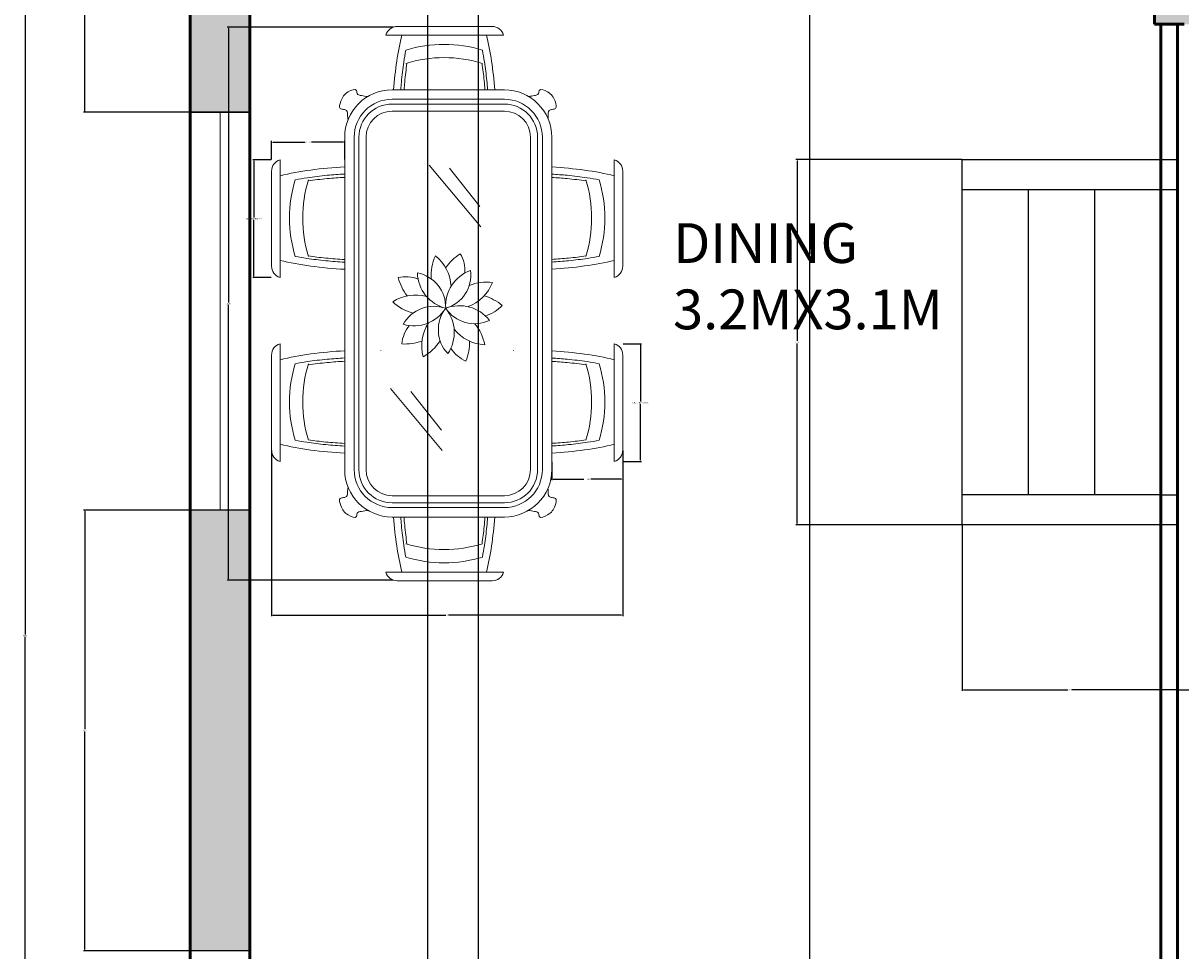
# Model space of a CAD drawing. Units: inches. Extents: x 3 to 380, y -485 to 60.
# Tile 4 of 8: x 3 to 177, y -270 to -130. Entities that reach past the tile are written whole.
import ezdxf

# ---------------------------------------------------------------- set-up
doc = ezdxf.new("R2010")
doc.units = ezdxf.units.IN
doc.header["$MEASUREMENT"] = 0
for name, color, linetype, lineweight in [('A-ANNO-DIMS', 2, 'Continuous', 18), ('A-AREA-IDEN', 7, 'Continuous', 25), ('A-FLOR-STRS', 7, 'Continuous', 25), ('A-FURN', 8, 'Continuous', 18), ('A-GLAZ', 4, 'Continuous', 18), ('A-WALL', 7, 'Continuous', 50), ('A-WALL-PATT', 252, 'Continuous', 13)]:
    doc.layers.add(name, color=color, linetype=linetype, lineweight=lineweight)
doc.styles.get("Standard").update_dxf_attribs({"font": 'arial.ttf'})
doc.dimstyles.get("Standard").update_dxf_attribs({"dimtxt": 0.18, "dimasz": 0.18, "dimexe": 0.18, "dimexo": 0.0625, "dimgap": 0.09, "dimtad": 0, "dimtih": 1, "dimtoh": 1, "dimdec": 0, "dimzin": 0, "dimdsep": 46, "dimlunit": 3, "dimtxsty": 'Standard', "dimcen": 0.09, "dimadec": 0, "dimazin": 0, "dimtfac": 1, "dimtdec": 0, "dimtofl": 0, "dimtmove": 0, "dimatfit": 3, "dimfxl": 1, "dimtolj": 1, "dimtzin": 0, "dimarcsym": 0})

# ---------------------------------------------------------------- blocks, each defined once
blk = doc.blocks.new('WIN-60X9')
for p, q in [((60, 9), (0, 9)), ((0, 9), (0, 0)), ((60, 0), (60, 9)), ((0, 4.5), (60, 4.5)), ((0, 0), (60, 0))]:
    blk.add_line(p, q)
blk = doc.blocks.new('DINING-CHAIR-A')
blk.add_line((9.42, 0), (9.42, 17.76))
blk.add_lwpolyline([(9.42, 17.76, -0.333667), (10.71, 16.04), (10.71, 1.72, -0.333667), (9.42, 0)], format="xyb")
for centre in [(-13.43, 8.97), (-11.43, 8.97)]:
    blk.add_arc(centre, 19.44, 342.7033, 17.2967)
at = {"extrusion": (0, 0, -1)}
for start_param, end_param in [(1.730141, 2.183659), (4.099527, 4.553045)]:
    blk.add_ellipse((-3.59, 8.97), major_axis=(-22.61, 0), ratio=0.345133, start_param=start_param, end_param=end_param, dxfattribs=at)
for points, knots in [([(0, 15.6), (0.78, 15.55), (1.55, 15.49), (3.34, 15.32), (4.35, 15.2), (5.94, 14.96), (6.54, 14.86), (7.13, 14.75)], [8.0160361, 8.0160361, 8.0160361, 8.0160361, 8.1227425, 8.1227425, 8.2664644, 8.2664644, 8.3579144, 8.3579144, 8.3579144, 8.3579144]), ([(0, 15.1), (0.78, 15.05), (1.55, 14.99), (3.29, 14.83), (4.25, 14.71), (5.18, 14.57)], [8.0160361, 8.0160361, 8.0160361, 8.0160361, 8.1227425, 8.1227425, 8.2598231, 8.2598231, 8.2598231, 8.2598231]), ([(5.15, 3.25), (4.3, 3.13), (3.43, 3.02), (1.7, 2.85), (0.86, 2.78), (0, 2.74)], [4.3081151, 4.3081151, 4.3081151, 4.3081151, 4.433179, 4.433179, 4.5503345, 4.5503345, 4.5503345, 4.5503345]), ([(7.13, 3.19), (6.56, 3.08), (5.98, 2.98), (4.47, 2.75), (3.51, 2.63), (1.7, 2.45), (0.86, 2.38), (0, 2.34)], [4.2084563, 4.2084563, 4.2084563, 4.2084563, 4.2962292, 4.2962292, 4.433179, 4.433179, 4.5503345, 4.5503345, 4.5503345, 4.5503345])]:
    blk.add_open_spline(points, degree=3, knots=knots)
blk = doc.blocks.new('DINING-CHAIR-B')
blk.add_line((1.29, 0), (1.29, 17.76))
blk.add_lwpolyline([(1.29, 17.76, 0.333667), (0, 16.04), (0, 1.72, 0.333667), (1.29, 0)], format="xyb")
for centre in [(22.14, 8.97), (24.14, 8.97)]:
    blk.add_arc(centre, 19.44, 162.7033, 197.2967)
for start_param, end_param in [(7.99879, 8.466844), (4.099527, 4.56758)]:
    blk.add_ellipse((14.3, 8.97), major_axis=(22.61, 0), ratio=0.345133, start_param=start_param, end_param=end_param)
for points, knots in [([(11.04, 15.61), (10.14, 15.57), (9.26, 15.5), (7.37, 15.32), (6.37, 15.2), (4.78, 14.96), (4.17, 14.86), (3.58, 14.75)], [8.0012444, 8.0012444, 8.0012444, 8.0012444, 8.1227425, 8.1227425, 8.2664644, 8.2664644, 8.3579144, 8.3579144, 8.3579144, 8.3579144]), ([(11.04, 15.11), (10.14, 15.07), (9.26, 15), (7.42, 14.83), (6.46, 14.71), (5.53, 14.57)], [8.0012444, 8.0012444, 8.0012444, 8.0012444, 8.1227425, 8.1227425, 8.2598231, 8.2598231, 8.2598231, 8.2598231]), ([(3.58, 3.19), (4.15, 3.08), (4.73, 2.98), (6.24, 2.75), (7.2, 2.63), (9.11, 2.44), (10.07, 2.37), (11.04, 2.32)], [4.2084563, 4.2084563, 4.2084563, 4.2084563, 4.2962292, 4.2962292, 4.433179, 4.433179, 4.5651263, 4.5651263, 4.5651263, 4.5651263]), ([(5.56, 3.25), (6.41, 3.13), (7.28, 3.02), (9.11, 2.84), (10.07, 2.77), (11.04, 2.72)], [4.3081151, 4.3081151, 4.3081151, 4.3081151, 4.433179, 4.433179, 4.5651263, 4.5651263, 4.5651263, 4.5651263])]:
    blk.add_open_spline(points, degree=3, knots=knots)
blk = doc.blocks.new('*D41')
at = {"layer": 'A-ANNO-DIMS', "color": 0, "lineweight": -2, "transparency": 16777216}
for p, q in [((93.19, -178.54), (95.97, -178.54)), ((95.79, -178.72), (95.79, -187.24)), ((95.79, -196.12), (95.79, -187.6)), ((93.19, -196.3), (95.97, -196.3))]:
    blk.add_line(p, q, dxfattribs=at)
at = {"layer": 'A-ANNO-DIMS', "color": 0, "transparency": 16777216}
for points in [[(95.76, -178.72), (95.82, -178.72), (95.79, -178.54)], [(95.76, -196.12), (95.82, -196.12), (95.79, -196.3)]]:
    blk.add_solid(points, dxfattribs=at)
at = {"layer": 'Defpoints', "color": 0, "transparency": 16777216}
for p in [(93.13, -178.54), (95.79, -178.54), (93.13, -196.3)]:
    blk.add_point(p, dxfattribs=at)
at = {"layer": 'A-ANNO-DIMS', "color": 0, "transparency": 16777216, "insert": (95.79, -187.42), "char_height": 0.18, "attachment_point": 5}
blk.add_mtext('\\A1;SIDE CHAIR A 18 TYP.', dxfattribs=at)
blk = doc.blocks.new('*D42')
at = {"layer": 'A-ANNO-DIMS', "color": 0, "lineweight": -2, "transparency": 16777216}
for p, q in [((82.42, -196.36), (82.42, -199.14)), ((93.13, -196.36), (93.13, -199.14)), ((82.6, -198.96), (87.25, -198.96)), ((92.95, -198.96), (88.29, -198.96))]:
    blk.add_line(p, q, dxfattribs=at)
at = {"layer": 'A-ANNO-DIMS', "color": 0, "transparency": 16777216}
for points in [[(82.6, -198.93), (82.6, -198.99), (82.42, -198.96)], [(92.95, -198.93), (92.95, -198.99), (93.13, -198.96)]]:
    blk.add_solid(points, dxfattribs=at)
at = {"layer": 'Defpoints', "color": 0, "transparency": 16777216}
for p in [(82.42, -196.3), (93.13, -196.3), (93.13, -198.96)]:
    blk.add_point(p, dxfattribs=at)
at = {"layer": 'A-ANNO-DIMS', "color": 0, "transparency": 16777216, "insert": (87.77, -198.96), "char_height": 0.18, "attachment_point": 5}
blk.add_mtext('\\A1;11 TYP.', dxfattribs=at)
blk = doc.blocks.new('*D43')
at = {"layer": 'A-ANNO-DIMS', "color": 0, "lineweight": -2, "transparency": 16777216}
for p, q in [((40.06, -150.79), (37.28, -150.79)), ((37.46, -150.97), (37.46, -159.49)), ((37.46, -168.37), (37.46, -159.86)), ((40.06, -168.55), (37.28, -168.55))]:
    blk.add_line(p, q, dxfattribs=at)
at = {"layer": 'A-ANNO-DIMS', "color": 0, "transparency": 16777216}
for points in [[(37.43, -150.97), (37.49, -150.97), (37.46, -150.79)], [(37.43, -168.37), (37.49, -168.37), (37.46, -168.55)]]:
    blk.add_solid(points, dxfattribs=at)
at = {"layer": 'Defpoints', "color": 0, "transparency": 16777216}
for p in [(37.46, -150.79), (40.12, -150.79), (40.12, -168.55)]:
    blk.add_point(p, dxfattribs=at)
at = {"layer": 'A-ANNO-DIMS', "color": 0, "transparency": 16777216, "insert": (37.46, -159.67), "char_height": 0.18, "attachment_point": 5}
blk.add_mtext('\\A1;SIDE CHAIR B 18 TYP.', dxfattribs=at)
blk = doc.blocks.new('*D44')
at = {"layer": 'A-ANNO-DIMS', "color": 0, "lineweight": -2, "transparency": 16777216}
for p, q in [((40.12, -150.73), (40.12, -147.95)), ((40.3, -148.13), (45.12, -148.13)), ((50.98, -148.13), (46.16, -148.13)), ((51.16, -150.73), (51.16, -147.95))]:
    blk.add_line(p, q, dxfattribs=at)
at = {"layer": 'A-ANNO-DIMS', "color": 0, "transparency": 16777216}
for points in [[(40.3, -148.1), (40.3, -148.16), (40.12, -148.13)], [(50.98, -148.1), (50.98, -148.16), (51.16, -148.13)]]:
    blk.add_solid(points, dxfattribs=at)
at = {"layer": 'Defpoints', "color": 0, "transparency": 16777216}
for p in [(51.16, -148.13), (40.12, -150.79), (51.16, -150.79)]:
    blk.add_point(p, dxfattribs=at)
at = {"layer": 'A-ANNO-DIMS', "color": 0, "transparency": 16777216, "insert": (45.64, -148.13), "char_height": 0.18, "attachment_point": 5}
blk.add_mtext('\\A1;11 TYP.', dxfattribs=at)
blk = doc.blocks.new('*D50')
at = {"layer": 'A-ANNO-DIMS', "color": 0, "lineweight": -2, "transparency": 16777216}
for p, q in [((27.78, 15.16), (2.76, 15.16)), ((2.94, 14.98), (2.94, -222.4)), ((2.94, -460.16), (2.94, -222.77)), ((27.78, -460.34), (2.76, -460.34))]:
    blk.add_line(p, q, dxfattribs=at)
at = {"layer": 'A-ANNO-DIMS', "color": 0, "transparency": 16777216}
for points in [[(2.91, 14.98), (2.97, 14.98), (2.94, 15.16)], [(2.91, -460.16), (2.97, -460.16), (2.94, -460.34)]]:
    blk.add_solid(points, dxfattribs=at)
at = {"layer": 'Defpoints', "color": 0, "transparency": 16777216}
for p in [(2.94, 15.16), (27.84, 15.16), (27.84, -460.34)]:
    blk.add_point(p, dxfattribs=at)
at = {"layer": 'A-ANNO-DIMS', "color": 0, "transparency": 16777216, "insert": (2.94, -222.59), "char_height": 0.18, "attachment_point": 5}
blk.add_mtext('\\A1;475.5', dxfattribs=at)
blk = doc.blocks.new('*D51')
at = {"layer": 'A-ANNO-DIMS', "color": 0, "lineweight": -2, "transparency": 16777216}
for p, q in [((151.9, 34.66), (379.92, 34.66)), ((379.74, 34.48), (379.74, -212.65)), ((379.74, -460.16), (379.74, -213.02)), ((354.9, -460.34), (379.92, -460.34))]:
    blk.add_line(p, q, dxfattribs=at)
at = {"layer": 'A-ANNO-DIMS', "color": 0, "transparency": 16777216}
for points in [[(379.71, 34.48), (379.77, 34.48), (379.74, 34.66)], [(379.71, -460.16), (379.77, -460.16), (379.74, -460.34)]]:
    blk.add_solid(points, dxfattribs=at)
at = {"layer": 'Defpoints', "color": 0, "transparency": 16777216}
for p in [(151.84, 34.66), (354.84, -460.34), (379.74, -460.34)]:
    blk.add_point(p, dxfattribs=at)
at = {"layer": 'A-ANNO-DIMS', "color": 0, "transparency": 16777216, "insert": (379.74, -212.84), "char_height": 0.18, "attachment_point": 5}
blk.add_mtext('\\A1;495', dxfattribs=at)
blk = doc.blocks.new('*D53')
at = {"layer": 'A-ANNO-DIMS', "color": 0, "lineweight": -2, "transparency": 16777216}
for p, q in [((36.78, 6.16), (11.76, 6.16)), ((11.94, 5.98), (11.94, -68.55)), ((11.94, -143.45), (11.94, -68.92)), ((36.78, -143.63), (11.76, -143.63))]:
    blk.add_line(p, q, dxfattribs=at)
at = {"layer": 'A-ANNO-DIMS', "color": 0, "transparency": 16777216}
for points in [[(11.91, 5.98), (11.97, 5.98), (11.94, 6.16)], [(11.91, -143.45), (11.97, -143.45), (11.94, -143.63)]]:
    blk.add_solid(points, dxfattribs=at)
at = {"layer": 'Defpoints', "color": 0, "transparency": 16777216}
for p in [(11.94, 6.16), (36.84, 6.16), (36.84, -143.63)]:
    blk.add_point(p, dxfattribs=at)
at = {"layer": 'A-ANNO-DIMS', "color": 0, "transparency": 16777216, "insert": (11.94, -68.73), "char_height": 0.18, "attachment_point": 5}
blk.add_mtext('\\A1;149.8', dxfattribs=at)
blk = doc.blocks.new('*D54')
at = {"layer": 'A-ANNO-DIMS', "color": 0, "lineweight": -2, "transparency": 16777216}
for p, q in [((36.78, -203.63), (11.76, -203.63)), ((11.94, -203.81), (11.94, -236.7)), ((11.94, -269.95), (11.94, -237.06)), ((36.78, -270.13), (11.76, -270.13))]:
    blk.add_line(p, q, dxfattribs=at)
at = {"layer": 'A-ANNO-DIMS', "color": 0, "transparency": 16777216}
for points in [[(11.91, -203.81), (11.97, -203.81), (11.94, -203.63)], [(11.91, -269.95), (11.97, -269.95), (11.94, -270.13)]]:
    blk.add_solid(points, dxfattribs=at)
at = {"layer": 'Defpoints', "color": 0, "transparency": 16777216}
for p in [(11.94, -203.63), (36.84, -203.63), (36.84, -270.13)]:
    blk.add_point(p, dxfattribs=at)
at = {"layer": 'A-ANNO-DIMS', "color": 0, "transparency": 16777216, "insert": (11.94, -236.88), "char_height": 0.18, "attachment_point": 5}
blk.add_mtext('\\A1;66.5', dxfattribs=at)
blk = doc.blocks.new('*D86')
at = {"layer": 'A-ANNO-DIMS', "color": 0, "lineweight": -2, "transparency": 16777216}
for p, q in [((176.84, -205.9), (176.84, -230.92)), ((209.34, -205.9), (209.34, -230.92)), ((177.02, -230.74), (192.77, -230.74)), ((209.16, -230.74), (193.41, -230.74))]:
    blk.add_line(p, q, dxfattribs=at)
at = {"layer": 'A-ANNO-DIMS', "color": 0, "transparency": 16777216}
for points in [[(177.02, -230.71), (177.02, -230.77), (176.84, -230.74)], [(209.16, -230.71), (209.16, -230.77), (209.34, -230.74)]]:
    blk.add_solid(points, dxfattribs=at)
at = {"layer": 'Defpoints', "color": 0, "transparency": 16777216}
for p in [(176.84, -205.84), (209.34, -205.84), (176.84, -230.74)]:
    blk.add_point(p, dxfattribs=at)
at = {"layer": 'A-ANNO-DIMS', "color": 0, "transparency": 16777216, "insert": (193.09, -230.74), "char_height": 0.18, "attachment_point": 5}
blk.add_mtext('\\A1;32.5', dxfattribs=at)
blk = doc.blocks.new('*D87')
at = {"layer": 'A-ANNO-DIMS', "color": 0, "lineweight": -2, "transparency": 16777216}
for p, q in [((144.34, -205.9), (144.34, -230.92)), ((176.84, -205.9), (176.84, -230.92)), ((144.52, -230.74), (160.27, -230.74)), ((176.66, -230.74), (160.91, -230.74))]:
    blk.add_line(p, q, dxfattribs=at)
at = {"layer": 'A-ANNO-DIMS', "color": 0, "transparency": 16777216}
for points in [[(144.52, -230.71), (144.52, -230.77), (144.34, -230.74)], [(176.66, -230.71), (176.66, -230.77), (176.84, -230.74)]]:
    blk.add_solid(points, dxfattribs=at)
at = {"layer": 'Defpoints', "color": 0, "transparency": 16777216}
for p in [(144.34, -205.84), (176.84, -205.84), (144.34, -230.74)]:
    blk.add_point(p, dxfattribs=at)
at = {"layer": 'A-ANNO-DIMS', "color": 0, "transparency": 16777216, "insert": (160.59, -230.74), "char_height": 0.18, "attachment_point": 5}
blk.add_mtext('\\A1;32.5', dxfattribs=at)
blk = doc.blocks.new('*D88')
at = {"layer": 'A-ANNO-DIMS', "color": 0, "lineweight": -2, "transparency": 16777216}
for p, q in [((144.28, -150.76), (119.26, -150.76)), ((119.44, -150.94), (119.44, -178.12)), ((119.44, -205.66), (119.44, -178.48)), ((144.28, -205.84), (119.26, -205.84))]:
    blk.add_line(p, q, dxfattribs=at)
at = {"layer": 'A-ANNO-DIMS', "color": 0, "transparency": 16777216}
for points in [[(119.41, -150.94), (119.47, -150.94), (119.44, -150.76)], [(119.41, -205.66), (119.47, -205.66), (119.44, -205.84)]]:
    blk.add_solid(points, dxfattribs=at)
at = {"layer": 'Defpoints', "color": 0, "transparency": 16777216}
for p in [(119.44, -150.76), (144.34, -150.76), (144.34, -205.84)]:
    blk.add_point(p, dxfattribs=at)
at = {"layer": 'A-ANNO-DIMS', "color": 0, "transparency": 16777216, "insert": (119.44, -178.3), "char_height": 0.18, "attachment_point": 5}
blk.add_mtext('\\A1;55.08', dxfattribs=at)
blk = doc.blocks.new('*D92')
at = {"layer": 'A-ANNO-DIMS', "color": 0, "lineweight": -2, "transparency": 16777216}
for p, q in [((36.84, -85.2), (36.84, -485.42)), ((63.65, -85.2), (63.65, -485.42)), ((37.02, -485.24), (49.87, -485.24)), ((63.47, -485.24), (50.62, -485.24))]:
    blk.add_line(p, q, dxfattribs=at)
at = {"layer": 'A-ANNO-DIMS', "color": 0, "transparency": 16777216}
for points in [[(37.02, -485.21), (37.02, -485.27), (36.84, -485.24)], [(63.47, -485.21), (63.47, -485.27), (63.65, -485.24)]]:
    blk.add_solid(points, dxfattribs=at)
at = {"layer": 'Defpoints', "color": 0, "transparency": 16777216}
for p in [(36.84, -85.14), (63.65, -85.14), (63.65, -485.24)]:
    blk.add_point(p, dxfattribs=at)
at = {"layer": 'A-ANNO-DIMS', "color": 0, "transparency": 16777216, "insert": (50.24, -485.24), "char_height": 0.18, "attachment_point": 5}
blk.add_mtext('\\A1;26.81', dxfattribs=at)
blk = doc.blocks.new('*D93')
at = {"layer": 'A-ANNO-DIMS', "color": 0, "lineweight": -2, "transparency": 16777216}
for p, q in [((71.32, -23.85), (71.32, -485.42)), ((121.32, -23.85), (121.32, -485.42)), ((71.5, -485.24), (95.92, -485.24)), ((121.14, -485.24), (96.72, -485.24))]:
    blk.add_line(p, q, dxfattribs=at)
at = {"layer": 'A-ANNO-DIMS', "color": 0, "transparency": 16777216}
for points in [[(71.5, -485.21), (71.5, -485.27), (71.32, -485.24)], [(121.14, -485.21), (121.14, -485.27), (121.32, -485.24)]]:
    blk.add_solid(points, dxfattribs=at)
at = {"layer": 'Defpoints', "color": 0, "transparency": 16777216}
for p in [(71.32, -23.79), (121.32, -23.79), (71.32, -485.24)]:
    blk.add_point(p, dxfattribs=at)
at = {"layer": 'A-ANNO-DIMS', "color": 0, "transparency": 16777216, "insert": (96.32, -485.24), "char_height": 0.18, "attachment_point": 5}
blk.add_mtext('\\A1;49.99', dxfattribs=at)
blk = doc.blocks.new('*D101')
at = {"layer": 'A-ANNO-DIMS', "color": 0, "lineweight": -2, "transparency": 16777216}
for p, q in [((40.12, -194.64), (40.12, -219.66)), ((93.13, -194.64), (93.13, -219.66)), ((40.3, -219.48), (66.4, -219.48)), ((92.95, -219.48), (66.84, -219.48))]:
    blk.add_line(p, q, dxfattribs=at)
at = {"layer": 'A-ANNO-DIMS', "color": 0, "transparency": 16777216}
for points in [[(40.3, -219.45), (40.3, -219.51), (40.12, -219.48)], [(92.95, -219.45), (92.95, -219.51), (93.13, -219.48)]]:
    blk.add_solid(points, dxfattribs=at)
at = {"layer": 'Defpoints', "color": 0, "transparency": 16777216}
for p in [(40.12, -194.58), (93.13, -194.58), (40.12, -219.48)]:
    blk.add_point(p, dxfattribs=at)
at = {"layer": 'A-ANNO-DIMS', "color": 0, "transparency": 16777216, "insert": (66.62, -219.48), "char_height": 0.18, "attachment_point": 5}
blk.add_mtext('\\A1;53', dxfattribs=at)
blk = doc.blocks.new('*D102')
at = {"layer": 'A-ANNO-DIMS', "color": 0, "lineweight": -2, "transparency": 16777216}
for p, q in [((58.46, -130.77), (33.44, -130.77)), ((33.62, -130.95), (33.62, -172.3)), ((33.62, -214.02), (33.62, -172.67)), ((58.46, -214.2), (33.44, -214.2))]:
    blk.add_line(p, q, dxfattribs=at)
at = {"layer": 'A-ANNO-DIMS', "color": 0, "transparency": 16777216}
for points in [[(33.59, -130.95), (33.65, -130.95), (33.62, -130.77)], [(33.59, -214.02), (33.65, -214.02), (33.62, -214.2)]]:
    blk.add_solid(points, dxfattribs=at)
at = {"layer": 'Defpoints', "color": 0, "transparency": 16777216}
for p in [(33.62, -130.77), (58.52, -130.77), (58.52, -214.2)]:
    blk.add_point(p, dxfattribs=at)
at = {"layer": 'A-ANNO-DIMS', "color": 0, "transparency": 16777216, "insert": (33.62, -172.49), "char_height": 0.18, "attachment_point": 5}
blk.add_mtext('\\A1;83.43', dxfattribs=at)

msp = doc.modelspace()

# ---------------------------------------------------------------- hatches: boundary and pattern name
at = {"layer": 'A-WALL-PATT'}
h = msp.add_hatch(color=256, dxfattribs=at)
h.dxf.hatch_style = 1
h.paths.add_polyline_path([(36.8404, 6.1643), (51.3404, 6.1643), (51.3404, 15.1643), (27.8404, 15.1643), (27.8404, -143.6318), (36.8404, -143.6318)])
h.paths.add_polyline_path([(125.8404, 10.6643), (125.8404, 15.1643), (111.3404, 15.1643), (111.3404, 6.1643), (125.8404, 6.1643)])
h.paths.add_polyline_path([(170.6358, 15.1643), (153.8404, 15.1643), (153.8404, 6.1643), (156.8404, 6.1643), (156.8404, -82.3357), (173.3404, -82.3357), (173.3404, -130.3357), (177.8404, -130.3357), (180.8404, -130.3357), (180.8404, -125.8357), (177.8404, -125.8357), (177.8404, -82.3357), (201.8404, -82.3357), (201.8404, -38.0857), (197.3404, -38.0857), (197.3404, -77.8357), (161.3404, -77.8357), (161.3404, 6.1643), (170.6358, 6.1643)])
h.paths.add_polyline_path([(241.3739, 15.1643), (194.6358, 15.1643), (194.6358, 6.1643), (241.3739, 6.1643)])
h.paths.add_polyline_path([(201.8404, 6.1643), (197.3404, 6.1643), (197.3404, -12.1977), (201.8404, -12.1977)], flags=17)
h.paths.add_polyline_path([(354.8404, 15.1643), (301.3739, 15.1643), (301.3739, 6.1643), (345.8404, 6.1643), (345.8404, -34.0336), (354.8404, -34.0336)])
h.paths.add_polyline_path([(354.8404, -94.0336), (345.8404, -94.0336), (345.8404, -159.3738), (354.8404, -159.3738)])
h.paths.add_polyline_path([(345.8404, -125.8357), (209.3404, -125.8357), (209.3404, -205.8357), (211.5904, -205.8357), (213.8404, -205.8357), (213.8404, -130.3357), (345.8404, -130.3357)])
h.paths.add_polyline_path([(36.8404, -203.6318), (27.8404, -203.6318), (27.8404, -270.1269), (36.8404, -270.1269)])
h.paths.add_polyline_path([(36.8404, -330.1269), (27.8404, -330.1269), (27.8404, -362.428), (57.3404, -362.428), (57.3404, -353.428), (36.8404, -353.428)])
h.paths.add_polyline_path([(177.8404, -331.3357), (180.8404, -331.3357), (180.8404, -326.8357), (173.3404, -326.8357), (173.3404, -353.428), (165.8404, -353.428), (165.8404, -362.428), (168.8404, -362.428), (168.8404, -451.3357), (168.8404, -460.3357), (231.8404, -460.3357), (231.8404, -451.3357), (177.8404, -451.3357)])
h.paths.add_polyline_path([(354.8404, -305.1003), (345.8404, -305.1003), (345.8404, -363.2829), (354.8404, -363.2829)])
h.paths.add_polyline_path([(345.8404, -326.8357), (213.8404, -326.8357), (213.8404, -312.8357), (211.5904, -312.8357), (209.3404, -312.8357), (209.3404, -331.3357), (345.8404, -331.3357)])
h.paths.add_polyline_path([(345.8404, -262.3357), (237.8404, -262.3357), (237.8404, -233.8357), (209.3404, -233.8357), (209.3404, -284.8357), (213.8404, -284.8357), (213.8404, -238.3357), (233.3404, -238.3357), (233.3404, -266.8357), (345.8404, -266.8357)])
h.paths.add_polyline_path([(354.8404, -219.3738), (345.8404, -219.3738), (345.8404, -281.1003), (354.8404, -281.1003)])

# ---------------------------------------------------------------- linework, layer by layer
at = {"layer": 'A-FLOR-STRS'}
for p, q in [((144.3404, -205.8357), (144.3404, -150.7599)), ((144.3404, -150.7599), (176.8404, -150.7599)), ((144.3404, -155.2599), (176.8404, -155.2599)), ((154.3404, -201.3357), (154.3404, -155.2599)), ((164.3404, -201.3357), (164.3404, -155.2599)), ((174.3404, -201.3357), (144.3404, -201.3357)), ((174.3404, -201.3357), (176.8404, -201.3357)), ((154.3404, -205.8357), (144.3404, -205.8357)), ((164.3404, -205.8357), (154.3404, -205.8357)), ((174.3404, -205.8357), (164.3404, -205.8357)), ((176.8404, -205.8357), (174.3404, -205.8357))]:
    msp.add_line(p, q, dxfattribs=at)
at = {"layer": 'A-FURN'}
for p, q in [((75.1318, -131.9654), (57.3752, -131.9654)), ((63.8848, -151.5902), (71.6802, -160.9281)), ((66.959, -152.0296), (71.5704, -157.8521)), ((56.6216, -179.614), (56.6216, -179.5632)), ((76.6251, -179.614), (76.6251, -179.5632)), ((58.0657, -185.3167), (65.8611, -194.6547)), ((61.14, -185.7561), (65.7513, -191.5786)), ((75.1318, -213.0049), (57.3752, -213.0049))]:
    msp.add_line(p, q, dxfattribs=at)
for points in [[(57.3752, -131.9654, -0.33366691), (59.094, -130.6747), (73.4129, -130.6747, -0.33366691), (75.1318, -131.9654)], [(57.3752, -213.0049, 0.33366691), (59.094, -214.2957), (73.4129, -214.2957, 0.33366691), (75.1318, -213.0049)]]:
    msp.add_lwpolyline(points, format="xyb", dxfattribs=at)
for points in [[(51.1567, -197.5243), (51.1567, -147.3879, -0.41421356), (58.3161, -140.2285), (75.2556, -140.2285, -0.41421356), (82.415, -147.3879), (82.415, -197.5243, -0.41421356), (75.2556, -204.6837), (58.3161, -204.6837, -0.41421356)], [(52.5886, -197.5243), (52.5886, -147.3879, -0.41421356), (58.3161, -141.6604), (75.2556, -141.6604, -0.41421356), (80.9831, -147.3879), (80.9831, -197.5243, -0.41421356), (75.2556, -203.2519), (58.3161, -203.2519, -0.41421356)], [(53.3045, -197.5243), (53.3045, -147.3879, -0.41421356), (58.3161, -142.3763), (75.2556, -142.3763, -0.41421356), (80.2672, -147.3879), (80.2672, -197.5243, -0.41421356), (75.2556, -202.5359), (58.3161, -202.5359, -0.41421356)], [(54.3784, -197.5243), (54.3784, -147.3879, -0.41421356), (58.3161, -143.4502), (75.2556, -143.4502, -0.41421356), (79.1933, -147.3879), (79.1933, -197.5243, -0.41421356), (75.2556, -201.462), (58.3161, -201.462, -0.41421356)]]:
    msp.add_lwpolyline(points, format="xyb", close=True, dxfattribs=at)
for centre, radius, start, end in [((66.1662, -152.8149), 19.4396, 72.703346, 107.296654), ((66.1662, -154.8162), 19.4396, 72.703346, 107.296654), ((70.8991, -168.2206), 6.712, 154.130103, 184.49315), ((61.0161, -170.1417), 6.1882, 2.132403, 51.601295), ((73.1708, -171.9366), 8.3447, 123.210515, 144.351409), ((64.1092, -167.5737), 5.1989, 356.508629, 30.24757), ((72.091, -172.8485), 5.7052, 109.776078, 183.515873), ((64.9428, -168.1434), 5.2599, 286.044681, 7.247269), ((60.3403, -173.6357), 5.1989, 68.508629, 102.24757), ((67.2899, -166.3658), 8.3447, 195.210516, 216.351409), ((61.1397, -173.0189), 5.2599, 358.044681, 79.24727), ((67.8235, -167.6745), 5.7052, 181.776079, 255.515873), ((67.641, -167.1367), 6.1882, 290.132404, 339.601296), ((72.5221, -175.9423), 6.712, 82.130102, 112.49315), ((61.8268, -177.371), 6.1882, 74.132404, 123.601295), ((63.0538, -167.378), 6.712, 226.130101, 256.49315), ((64.6014, -178.1425), 5.2599, 70.044681, 151.247269), ((68.489, -178.506), 5.7052, 37.776078, 111.515873), ((69.69, -179.2512), 8.3447, 51.210515, 72.351409), ((71.0392, -169.2848), 5.1989, 284.508629, 318.24757), ((61.584, -170.1343), 5.7052, 253.776078, 327.515873), ((70.544, -176.4335), 5.2599, 142.044681, 223.24727), ((70.755, -170.2537), 5.2599, 214.044681, 295.24727), ((61.9953, -176.8286), 5.7052, 325.776078, 39.515873), ((64.941, -179.0934), 5.1989, 140.508629, 174.247571), ((68.9528, -178.8339), 6.1882, 146.132404, 195.601296), ((72.5462, -172.5088), 6.1882, 218.132404, 267.601295), ((65.6798, -179.872), 6.712, 10.130102, 40.49315), ((60.1744, -170.2375), 8.3447, 267.210515, 288.351409), ((59.8281, -174.579), 6.712, 298.130102, 328.493151), ((61.6578, -178.2011), 8.3447, 339.210516, 0.351408), ((71.5533, -176.4044), 5.1989, 212.508629, 246.24757), ((66.1662, -190.1542), 19.4396, 252.703346, 287.296654), ((66.1662, -192.1555), 19.4396, 252.703346, 287.296654)]:
    msp.add_arc(centre, radius, start, end, dxfattribs=at)
at = {"layer": 'A-FURN', "extrusion": (0, 0, -1)}
for start_param, end_param in [(4.92378376, 5.32525145), (0.95793386, 1.35940155)]:
    msp.add_ellipse((66.1662, -144.9735), major_axis=(0, 22.6145), ratio=0.34513274, start_param=start_param, end_param=end_param, dxfattribs=at)
at = {"layer": 'A-FURN'}
for start_param, end_param in [(8.06274752, 8.4668441), (4.09952651, 4.5036231)]:
    msp.add_ellipse((66.1662, -199.9968), major_axis=(0, 22.6145), ratio=0.34513274, start_param=start_param, end_param=end_param, dxfattribs=at)
for points, knots in [([(59.6119, -140.2285), (59.6412, -139.8398), (59.6741, -139.4535), (59.808, -138.0445), (59.9309, -137.0402), (60.1711, -135.4496), (60.2742, -134.8441), (60.3864, -134.2544)], [8.069029084, 8.069029084, 8.069029084, 8.069029084, 8.122742487, 8.122742487, 8.266464386, 8.266464386, 8.357914365, 8.357914365, 8.357914365, 8.357914365]), ([(71.9459, -134.2544), (72.0537, -134.8204), (72.153, -135.4009), (72.3844, -136.9183), (72.5038, -137.8725), (72.6454, -139.3033), (72.6855, -139.7642), (72.7205, -140.2285)], [4.208456323, 4.208456323, 4.208456323, 4.208456323, 4.296229184, 4.296229184, 4.433179016, 4.433179016, 4.497341533, 4.497341533, 4.497341533, 4.497341533]), ([(60.1126, -140.2285), (60.1419, -139.8398), (60.1747, -139.4535), (60.3042, -138.0919), (60.4203, -137.1331), (60.5582, -136.2031)], [8.069029084, 8.069029084, 8.069029084, 8.069029084, 8.122742487, 8.122742487, 8.259823146, 8.259823146, 8.259823146, 8.259823146]), ([(71.879, -136.235), (72.0044, -137.084), (72.1116, -137.9571), (72.2448, -139.3033), (72.285, -139.7642), (72.32, -140.2285)], [4.308115056, 4.308115056, 4.308115056, 4.308115056, 4.433179016, 4.433179016, 4.497341533, 4.497341533, 4.497341533, 4.497341533]), ([(54.6403, -141.2442), (54.3341, -141.2104), (53.7825, -141.1355), (52.9591, -140.9622), (53.0313, -139.8809), (51.2109, -140.689), (50.6701, -141.5307), (50.1773, -143.1168), (50.9782, -143.1586), (51.6314, -143.3398), (51.5663, -144.098), (51.6293, -144.578), (51.6621, -144.7457)], [26.59661158, 26.59661158, 26.59661158, 26.59661158, 52.77132907, 71.89490479, 86.11792846, 121.95473397, 172.04851004, 202.47617351, 216.69185485, 230.01003031, 254.63564309, 268.76794379, 268.76794379, 268.76794379, 268.76794379]), ([(78.9134, -141.2334), (79.1905, -141.2013), (79.7135, -141.1277), (80.4996, -140.9622), (80.4275, -139.8809), (82.2478, -140.689), (82.7886, -141.5307), (83.2814, -143.1168), (82.4806, -143.1586), (81.8274, -143.3398), (81.8858, -144.0201), (81.8447, -144.4439), (81.8294, -144.552)], [29.29082505, 29.29082505, 29.29082505, 29.29082505, 52.77132907, 71.89490479, 86.11792846, 121.95473397, 172.04851004, 202.47617351, 216.69185485, 230.01003031, 254.63564309, 263.41939686, 263.41939686, 263.41939686, 263.41939686]), ([(54.6663, -203.6836), (54.3522, -203.7177), (53.7927, -203.7929), (52.9591, -203.9684), (53.0313, -205.0496), (51.2109, -204.2416), (50.6701, -203.3999), (50.1773, -201.8138), (50.9782, -201.772), (51.6314, -201.5908), (51.5658, -200.8275), (51.6305, -200.344), (51.6645, -200.1726)], [25.85415121, 25.85415121, 25.85415121, 25.85415121, 52.77132907, 71.89490479, 86.11792846, 121.95473397, 172.04851004, 202.47617351, 216.69185485, 230.01003031, 254.63564309, 269.11298795, 269.11298795, 269.11298795, 269.11298795]), ([(78.8874, -203.6942), (79.1725, -203.7267), (79.7034, -203.8008), (80.4996, -203.9684), (80.4275, -205.0496), (82.2478, -204.2416), (82.7886, -203.3999), (83.2814, -201.8138), (82.4806, -201.772), (81.8274, -201.5908), (81.8863, -200.905), (81.8438, -200.4772), (81.8274, -200.3648)], [28.55667014, 28.55667014, 28.55667014, 28.55667014, 52.77132907, 71.89490479, 86.11792846, 121.95473397, 172.04851004, 202.47617351, 216.69185485, 230.01003031, 254.63564309, 263.79289499, 263.79289499, 263.79289499, 263.79289499]), ([(59.6075, -204.6837), (59.6379, -205.0921), (59.6722, -205.4978), (59.808, -206.9258), (59.9309, -207.9302), (60.1711, -209.5208), (60.2742, -210.1263), (60.3864, -210.716)], [8.066351515, 8.066351515, 8.066351515, 8.066351515, 8.122742487, 8.122742487, 8.266464386, 8.266464386, 8.357914365, 8.357914365, 8.357914365, 8.357914365]), ([(60.1082, -204.6837), (60.1386, -205.0921), (60.1729, -205.4978), (60.3042, -206.8785), (60.4203, -207.8373), (60.5582, -208.7673)], [8.066351515, 8.066351515, 8.066351515, 8.066351515, 8.122742487, 8.122742487, 8.259823146, 8.259823146, 8.259823146, 8.259823146]), ([(71.879, -208.7354), (72.0044, -207.8863), (72.1116, -207.0133), (72.2467, -205.648), (72.2883, -205.1677), (72.3243, -204.6837)], [4.308115056, 4.308115056, 4.308115056, 4.308115056, 4.433179016, 4.433179016, 4.500019108, 4.500019108, 4.500019108, 4.500019108]), ([(71.9459, -210.716), (72.0537, -210.15), (72.153, -209.5695), (72.3844, -208.0521), (72.5038, -207.0979), (72.6473, -205.648), (72.6888, -205.1677), (72.7249, -204.6837)], [4.208456323, 4.208456323, 4.208456323, 4.208456323, 4.296229184, 4.296229184, 4.433179016, 4.433179016, 4.500019108, 4.500019108, 4.500019108, 4.500019108])]:
    msp.add_open_spline(points, degree=3, knots=knots, dxfattribs=at)
at = {"layer": 'A-WALL'}
for p, q in [((27.8404, 15.1643), (27.8404, -460.3357)), ((36.8404, 6.1643), (36.8404, -353.428)), ((173.3404, -82.3357), (173.3404, -130.3357)), ((177.8404, -130.3357), (173.3404, -130.3357)), ((174.3404, -130.3357), (174.3404, -326.8357)), ((176.8404, -130.3357), (176.8404, -326.8357))]:
    msp.add_line(p, q, dxfattribs=at)

# ---------------------------------------------------------------- block references
at = {"layer": 'A-FURN'}
for name, p in [('DINING-CHAIR-B', (40.121, -168.5513)), ('DINING-CHAIR-A', (82.415, -168.5513)), ('DINING-CHAIR-B', (40.121, -196.297)), ('DINING-CHAIR-A', (82.415, -196.297))]:
    msp.add_blockref(name, p, dxfattribs=at)
at = {"layer": 'A-GLAZ', "rotation": 270}
msp.add_blockref('WIN-60X9', (27.84, -143.6319), dxfattribs=at)

# ---------------------------------------------------------------- texts
at = {"layer": 'A-AREA-IDEN', "insert": (100.7067, -160.3585), "char_height": 6, "attachment_point": 1}
msp.add_mtext('DINING\\P3.2MX3.1M', dxfattribs=at)

# ---------------------------------------------------------------- dimensions: what is measured, and where the dimension line sits
at = {"layer": 'A-ANNO-DIMS'}
for base, p1, p2, angle, override, picture, middle in [((379.7404, -460.3357), (151.8404, 34.6643), (354.8404, -460.3357), 90, {"dimdec": 0, "dimlfac": 1, "dimrnd": 0, "dimzin": 0, "dimdsep": 46, "dimlunit": 2}, '*D51', (379.7404, -212.8357)), ((2.9404, 15.1643), (27.8404, -460.3357), (27.8404, 15.1643), 90, {"dimdec": 1, "dimlfac": 1, "dimrnd": 0, "dimzin": 0, "dimdsep": 46, "dimlunit": 2}, '*D50', (2.9404, -222.5857)), ((11.9404, 6.1643), (36.8404, -143.6318), (36.8404, 6.1643), 90, {"dimdec": 1, "dimlfac": 1, "dimrnd": 0, "dimzin": 0, "dimdsep": 46, "dimlunit": 2}, '*D53', (11.9404, -68.7338)), ((33.6207, -130.7688), (58.5207, -214.2016), (58.5207, -130.7688), 90, {"dimdec": 2, "dimlfac": 1, "dimrnd": 0, "dimzin": 0, "dimdsep": 46, "dimlunit": 2}, '*D102', (33.6207, -172.4852)), ((119.4404, -150.7599), (144.3404, -205.8357), (144.3404, -150.7599), 90, {"dimdec": 2, "dimlfac": 1, "dimrnd": 0, "dimzin": 0, "dimdsep": 46, "dimlunit": 2}, '*D88', (119.4404, -178.2978)), ((40.1211, -219.4779), (93.1256, -194.5779), (40.1211, -194.5779), 180, {"dimdec": 0, "dimlfac": 1, "dimrnd": 0, "dimzin": 0, "dimdsep": 46, "dimlunit": 2}, '*D101', (66.6234, -219.4779)), ((11.9404, -203.6318), (36.8404, -270.1269), (36.8404, -203.6318), 90, {"dimdec": 1, "dimlfac": 1, "dimrnd": 0, "dimzin": 0, "dimdsep": 46, "dimlunit": 2}, '*D54', (11.9404, -236.8793)), ((144.3404, -230.7357), (176.8404, -205.8357), (144.3404, -205.8357), 180, {"dimdec": 1, "dimlfac": 1, "dimrnd": 0, "dimzin": 0, "dimdsep": 46, "dimlunit": 2}, '*D87', (160.5904, -230.7357)), ((176.8404, -230.7357), (209.3404, -205.8357), (176.8404, -205.8357), 180, {"dimdec": 1, "dimlfac": 1, "dimrnd": 0, "dimzin": 0, "dimdsep": 46, "dimlunit": 2}, '*D86', (193.0904, -230.7357))]:
    dim = msp.add_linear_dim(base=base, p1=p1, p2=p2, angle=angle, dimstyle='Standard', override=override, dxfattribs=at)
    dim.commit()
    dim.dimension.update_dxf_attribs({"geometry": picture, "text_midpoint": middle})
for base, p1, p2, picture, middle in [((71.3212, -485.2357), (121.3159, -23.7901), (71.3212, -23.7901), '*D93', (96.3185, -485.2357)), ((63.6489, -485.2357), (36.8404, -85.1388), (63.6489, -85.1388), '*D92', (50.2446, -485.2357))]:
    dim = msp.add_linear_dim(base=base, p1=p1, p2=p2, dimstyle='Standard', override={"dimdec": 2, "dimlfac": 1, "dimrnd": 0, "dimzin": 0, "dimdsep": 46, "dimlunit": 2}, dxfattribs=at)
    dim.commit()
    dim.dimension.update_dxf_attribs({"geometry": picture, "text_midpoint": middle})
for base, p1, p2, picture, middle in [((51.1567, -148.1309), (40.1211, -150.7944), (51.1567, -150.7944), '*D44', (45.6389, -148.1309)), ((93.1256, -198.9603), (82.415, -196.2968), (93.1256, -196.2968), '*D42', (87.7703, -198.9603))]:
    dim = msp.add_linear_dim(base=base, p1=p1, p2=p2, text='<> TYP.', dimstyle='Standard', override={"dimdec": 0, "dimlfac": 1, "dimrnd": 0, "dimzin": 0, "dimdsep": 46, "dimlunit": 2}, dxfattribs=at)
    dim.commit()
    dim.dimension.update_dxf_attribs({"geometry": picture, "text_midpoint": middle})
for base, p1, p2, text, picture, middle in [((37.4576, -150.7944), (40.1211, -168.5511), (40.1211, -150.7944), 'SIDE CHAIR B <> TYP.', '*D43', (37.4576, -159.6727)), ((95.7891, -178.5401), (93.1256, -196.2968), (93.1256, -178.5401), 'SIDE CHAIR A <> TYP.', '*D41', (95.7891, -187.4185))]:
    dim = msp.add_linear_dim(base=base, p1=p1, p2=p2, angle=90, text=text, dimstyle='Standard', override={"dimdec": 0, "dimlfac": 1, "dimrnd": 0, "dimzin": 0, "dimdsep": 46, "dimlunit": 2}, dxfattribs=at)
    dim.commit()
    dim.dimension.update_dxf_attribs({"geometry": picture, "text_midpoint": middle})

doc.saveas('drawing.dxf')
